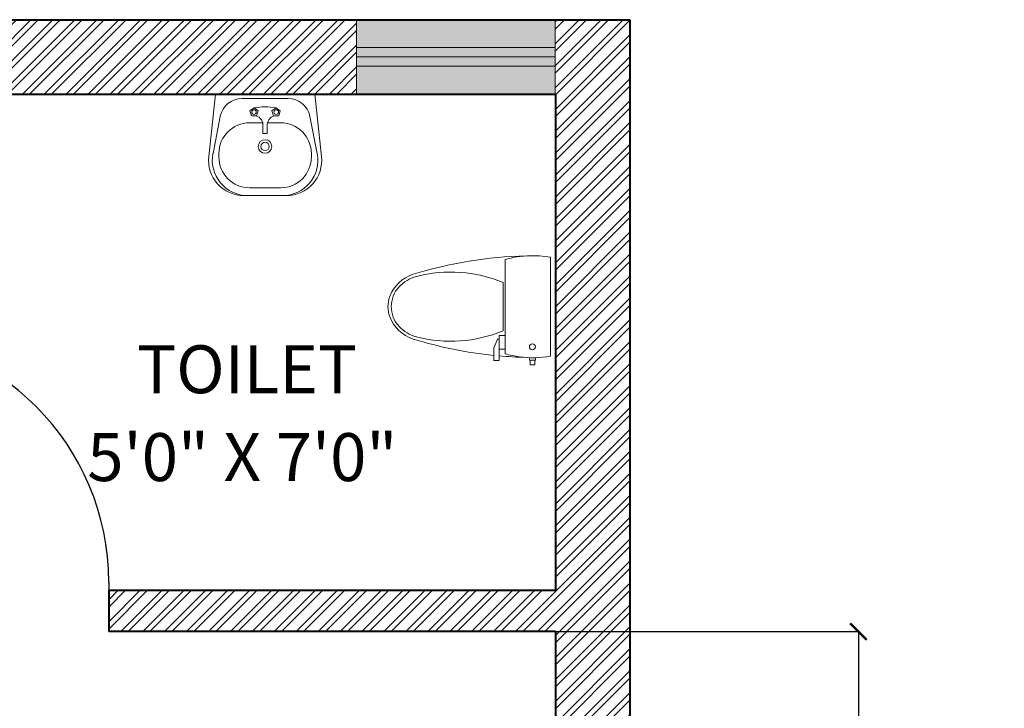
# Model space of a CAD drawing. Units: inches. Extents: x 528 to 2520, y -151 to 1354.
# Tile 41 of 41: x 2383 to 2502, y 815 to 898. Entities that reach past the tile are written whole.
import ezdxf

# ---------------------------------------------------------------- set-up
doc = ezdxf.new("R2010")
doc.units = ezdxf.units.IN
doc.header["$MEASUREMENT"] = 0
for name, color, linetype, lineweight in [('A-ANNO-DIMS', 2, 'Continuous', 18), ('A-AREA-IDEN', 7, 'Continuous', 18), ('A-Door', 150, 'Continuous', 25), ('A-ELEV-PROJ', 8, 'Continuous', 13), ('A-FLOR-FIXT', 9, 'Continuous', 18), ('A-WALL-PATT', 6, 'Continuous', 13), ('walls', 7, 'Continuous', 40), ('WINDOWS', 2, 'Continuous', 20)]:
    doc.layers.add(name, color=color, linetype=linetype, lineweight=lineweight)
doc.layers.add('A-GLAZ-PATT', color=152, linetype='Continuous', lineweight=13, true_color=0x2776bb)
doc.styles.get("Standard").update_dxf_attribs({"font": 'arial.ttf'})
doc.dimstyles.get("Standard").update_dxf_attribs({"dimtxt": 6, "dimasz": 2, "dimexe": 0.18, "dimexo": 0.0625, "dimgap": 0.09, "dimtad": 0, "dimtih": 1, "dimtoh": 1, "dimdec": 1, "dimzin": 0, "dimdsep": 46, "dimlunit": 3, "dimtxsty": 'Standard', "dimblk": 'ARCHTICK', "dimcen": 0.09, "dimadec": 0, "dimazin": 0, "dimtfac": 1, "dimtdec": 1, "dimtofl": 0, "dimtmove": 0, "dimatfit": 3, "dimfxl": 1, "dimtolj": 1, "dimtzin": 0, "dimarcsym": 0})

# ---------------------------------------------------------------- blocks, each defined once
blk = doc.blocks.new('toilet-7')
at = {"color": 0, "linetype": 'ByBlock'}
for p, q in [((0.2097, -0.02), (-0.2097, -0.02)), ((0.2151, -0.0677), (0.2097, -0.02)), ((0.2151, -0.1171), (0.2151, -0.0677)), ((-0.2457, -0.0874), (-0.2457, -0.1068)), ((-0.2457, -0.0874), (-0.2257, -0.0874)), ((-0.2457, -0.1068), (-0.2257, -0.1068)), ((-0.2257, -0.0846), (-0.2257, -0.1096)), ((-0.2257, -0.0846), (-0.2157, -0.0846)), ((-0.2257, -0.1096), (-0.2154, -0.1096)), ((0.2099, -0.164), (0.2151, -0.1171)), ((0.1991, -0.2124), (0.2099, -0.164)), ((-0.1213, -0.2374), (-0.2278, -0.2374)), ((-0.2278, -0.2374), (-0.2278, -0.2599)), ((0.1991, -0.2124), (-0.1991, -0.2124)), ((-0.1803, -0.2374), (-0.1803, -0.2124)), ((-0.1759, -0.2599), (-0.1379, -0.2451)), ((-0.1379, -0.2451), (-0.1379, -0.2374)), ((-0.1213, -0.2374), (-0.1213, -0.2124)), ((-0.1023, -0.2212), (0.1023, -0.2212)), ((-0.1759, -0.2599), (-0.2278, -0.2599))]:
    blk.add_line(p, q, dxfattribs=at)
blk.add_circle((-0.1696, -0.0971), 0.0125, dxfattribs=at)
for centre, radius, start, end in [((0.2244, -0.0924), 0.4402, 170.5377, 187.7399), ((1.517, -0.087), 1.7318, 181.2224, 184.9822), ((-1.517, -0.087), 1.7318, 342.7523, 358.7776), ((0.2244, -0.0924), 0.4402, 187.7399, 195.822), ((0.4258, -0.4413), 0.5721, 157.3737, 194.7786), ((-0.4258, -0.4413), 0.5721, 345.2214, 22.6263), ((1.517, -0.087), 1.7318, 185.7323, 197.2477), ((0.0116, -0.5544), 0.1554, 197.2477, 249.5476), ((0.0221, -0.5478), 0.1546, 194.7786, 226.8543), ((-0.0116, -0.5544), 0.1554, 290.4524, 342.7523), ((-0.0221, -0.5478), 0.1546, 313.1457, 345.2214), ((0, -0.5713), 0.1223, 226.8543, 313.1457), ((0, -0.5854), 0.1223, 249.5476, 290.4524)]:
    blk.add_arc(centre, radius, start, end, dxfattribs=at)
blk = doc.blocks.new('BASIN-WITH-TAP')
for p, q in [((0.84, 12.27), (0.02, 4.73)), ((12.84, 12.27), (0.84, 12.27)), ((12.84, 12.27), (13.66, 4.73)), ((9.64, 11.73), (4.05, 11.73)), ((1.43, 9.58), (0.55, 5.09)), ((5, 10.24), (5.51, 10.61)), ((5.2, 9.64), (5, 10.24)), ((5.24, 10.1), (5.2, 10.1)), ((5.24, 9.64), (5.51, 9.64)), ((5.51, 10.61), (6.02, 10.24)), ((6.02, 10.24), (5.82, 9.64)), ((8.18, 10.61), (7.67, 10.24)), ((7.67, 10.24), (7.86, 9.64)), ((8.68, 10.24), (8.18, 10.61)), ((8.49, 9.64), (8.18, 9.64)), ((8.44, 10.1), (8.49, 10.1)), ((8.49, 9.64), (8.68, 10.24)), ((12.26, 9.58), (13.14, 5.09)), ((4.98, 8.8), (6.58, 8.8)), ((6.58, 8.31), (6.58, 8.58)), ((8.71, 8.8), (7.11, 8.8)), ((7.11, 8.31), (7.11, 8.58)), ((6.58, 7.51), (6.58, 8.31)), ((6.58, 7.51), (7.11, 7.51)), ((7.11, 7.51), (7.11, 8.31)), ((1.24, 4.67), (1.24, 5.07)), ((12.44, 4.67), (12.44, 5.07)), ((4.73, 0), (8.96, 0)), ((6.84, 0.93), (4.98, 0.93)), ((6.84, 0.93), (8.71, 0.93))]:
    blk.add_line(p, q)
for centre, radius in [((5.5, 10.1), 0.277), ((8.19, 10.1), 0.277), ((6.84, 5.94), 0.821), ((6.84, 5.94), 0.507)]:
    blk.add_circle(centre, radius)
for centre, radius, start, end in [((4.05, 9.07), 2.67, 90, 168.8773), ((6.84, 4.01), 6.73, 78.5788, 101.4212), ((9.64, 9.07), 2.67, 11.1227, 90), ((5.51, 8.58), 1.07, 0, 90), ((8.18, 8.58), 1.07, 90, 180), ((4.98, 5.07), 3.73, 90, 180), ((8.71, 5.07), 3.73, 0, 90), ((4.73, 4.27), 4.27, 168.8773, 270), ((8.96, 4.27), 4.27, 270, 11.1227), ((4.27, 4.27), 4.27, 173.7966, 270), ((4.98, 4.67), 3.73, 180, 270), ((8.71, 4.67), 3.73, 270, 0), ((9.42, 4.27), 4.27, 270, 6.2034)]:
    blk.add_arc(centre, radius, start, end)
blk = doc.blocks.new('DOOR-SWING-30')
for p, q in [((0, 6), (0, 0)), ((30, 6), (30, 0))]:
    blk.add_line(p, q)
blk.add_lwpolyline([(0, 6), (0, 36), (1.75, 36), (1.75, 6)], close=True)
blk.add_arc((0, 6), 30, 0, 90)
blk = doc.blocks.new('WINDOW-24x9-PLAN')
for p, q in [((0, 5.63), (24, 5.63)), ((0, 4.5), (24, 4.5)), ((0, 3.37), (24, 3.37))]:
    blk.add_line(p, q)
blk.add_lwpolyline([(0, 9), (24, 9), (24, 0), (0, 0)], close=True)
blk = doc.blocks.new('_ArchTick')
at = {"color": 0, "linetype": 'ByBlock', "const_width": 0.15}
blk.add_lwpolyline([(-0.5, -0.5), (0.5, 0.5)], dxfattribs=at)
blk = doc.blocks.new('*D98')
at = {"layer": 'A-ANNO-DIMS', "color": 0, "lineweight": -2, "transparency": 16777216}
for p, q in [((2448.07, 823.94), (2484.84, 823.94)), ((2484.66, 823.94), (2484.66, 791.26)), ((2484.66, 752.2), (2484.66, 784.88)), ((2457.07, 752.2), (2484.84, 752.2))]:
    blk.add_line(p, q, dxfattribs=at)
at = {"layer": 'Defpoints', "color": 0, "transparency": 16777216}
for p in [(2448.01, 823.94), (2484.66, 823.94), (2457.01, 752.2)]:
    blk.add_point(p, dxfattribs=at)
at = {"layer": 'A-ANNO-DIMS', "color": 0, "lineweight": -2, "transparency": 16777216, "xscale": 2, "yscale": 2, "zscale": 2}
for p, rotation in [((2484.66, 823.94), 90), ((2484.66, 752.2), 270)]:
    blk.add_blockref('_ArchTick', p, dxfattribs=dict(at, rotation=rotation))
at = {"layer": 'A-ANNO-DIMS', "color": 0, "transparency": 16777216, "insert": (2484.66, 788.07), "char_height": 6, "attachment_point": 5}
blk.add_mtext('\\A1;5\'-11 1/2"', dxfattribs=at)

msp = doc.modelspace()

# ---------------------------------------------------------------- hatches: boundary and pattern name
at = {"layer": 'A-GLAZ-PATT'}
h = msp.add_hatch(color=256, dxfattribs=at)
h.dxf.hatch_style = 1
h.paths.add_polyline_path([(2447.97, 894.57), (2423.97, 894.57), (2423.97, 893.44), (2447.97, 893.44)])
h.paths.add_polyline_path([(2447.97, 893.44), (2423.97, 893.44), (2423.97, 892.31), (2447.97, 892.31)])
h.paths.add_polyline_path([(2447.97, 897.94), (2423.97, 897.94), (2423.97, 894.57), (2447.97, 894.57)])
h.paths.add_polyline_path([(2447.97, 892.31), (2423.97, 892.31), (2423.97, 888.94), (2447.97, 888.94)])
at = {"layer": 'A-WALL-PATT'}
h = msp.add_hatch(dxfattribs=at)
h.set_pattern_fill('ANSI32', color=256, scale=5)
h.set_pattern_definition([(45, (1571.3155, -419.1643), (-1.3258252, 1.3258252), []), (45, (1572.1993, -419.1643), (-1.3258252, 1.3258252), [])])
h.paths.add_polyline_path([(2167.01, 744.69), (2158.01, 744.69), (2158.01, 549.94), (2169.56, 549.94), (2174.56, 549.94), (2174.56, 554.94), (2167.01, 554.94), (2167.01, 662.94), (2263.01, 662.94), (2263.01, 667.94), (2263.01, 686.94), (2269.01, 686.94), (2269.01, 691.94), (2258.01, 691.94), (2258.01, 667.94), (2167.01, 667.94)])
h.paths.add_polyline_path([(2260.02, 554.94), (2222.56, 554.94), (2222.56, 549.94), (2260.02, 549.94)])
h.paths.add_polyline_path([(2457.01, 752.2), (2448.01, 752.2), (2448.01, 691.94), (2358.01, 691.94), (2358.01, 686.94), (2448.01, 686.94), (2448.01, 554.94), (2358.01, 554.94), (2358.01, 549.94), (2448.01, 549.94), (2448.01, 405.94), (2406.01, 405.94), (2406.01, 396.94), (2457.01, 396.94)])
h.paths.add_polyline_path([(2457.01, 897.94), (2447.97, 897.94), (2447.97, 888.94), (2448.01, 888.94), (2448.01, 828.94), (2394.01, 828.94), (2394.01, 823.94), (2448.01, 823.94), (2448.01, 800.2), (2457.01, 800.2)])
h.paths.add_polyline_path([(2423.97, 897.94), (2359.01, 897.94), (2359.01, 828.94), (2355.58, 828.94), (2355.58, 823.94), (2364.01, 823.94), (2364.01, 829.94), (2364.01, 888.94), (2423.97, 888.94)])
h.paths.add_polyline_path([(2256.01, 897.94), (2191.01, 897.94), (2191.01, 888.94), (2251.01, 888.94), (2251.01, 828.94), (2251.01, 823.94), (2256.01, 823.94), (2256.01, 829.08)])
h.paths.add_polyline_path([(2167.01, 888.94), (2167.01, 897.94), (2158.01, 897.94), (2158.01, 792.69), (2167.01, 792.69), (2167.01, 823.94), (2221.01, 823.94), (2221.01, 828.94), (2167.01, 828.94)])
h.paths.add_polyline_path([(2316.01, 549.94), (2316.01, 554.94), (2296.02, 554.94), (2296.02, 549.94), (2311.01, 549.94), (2311.01, 455.12), (2316.01, 455.12)])
h.paths.add_polyline_path([(2311.01, 549.94), (2299.01, 549.94), (2299.01, 545.95), (2302.05, 545.95), (2302.05, 542.51), (2305.75, 542.51), (2305.75, 538.08), (2311.01, 538.08)], flags=17)
h.paths.add_polyline_path([(2358.01, 405.94), (2316.01, 405.94), (2316.01, 413.12), (2311.01, 413.12), (2311.01, 396.94), (2358.01, 396.94)])

# ---------------------------------------------------------------- linework, layer by layer
at = {"layer": 'A-ELEV-PROJ'}
msp.add_line((2457.01, 360.94), (2457.01, 897.94), dxfattribs=at)
at = {"layer": 'walls'}
for p, q in [((2359.01, 897.94), (2457.01, 897.94)), ((2457.01, 897.94), (2457.01, 396.94)), ((2364.01, 888.94), (2448.01, 888.94)), ((2448.01, 888.94), (2448.01, 828.94)), ((2394.01, 828.94), (2448.01, 828.94)), ((2394.01, 828.94), (2394.01, 823.94)), ((2448.01, 823.94), (2394.01, 823.94)), ((2448.01, 823.94), (2448.01, 691.94))]:
    msp.add_line(p, q, dxfattribs=at)

# ---------------------------------------------------------------- block references
at = {"layer": 'A-Door'}
msp.add_blockref('DOOR-SWING-30', (2364.01, 823.94), dxfattribs=at)
at = {"layer": 'A-FLOR-FIXT'}
msp.add_blockref('BASIN-WITH-TAP', (2406.07, 876.67), dxfattribs=at)
at = {"layer": 'A-FLOR-FIXT', "xscale": -28.60654769571749, "yscale": 28.60654769571749, "zscale": 28.60654769571749, "rotation": 270}
msp.add_blockref('toilet-7', (2448.01, 863.24), dxfattribs=at)
at = {"layer": 'WINDOWS'}
msp.add_blockref('WINDOW-24x9-PLAN', (2423.97, 888.94), dxfattribs=at)

# ---------------------------------------------------------------- texts
at = {"layer": 'A-AREA-IDEN'}
for s, height, p in [('TOILET', 5.793, (2397.43, 852.77)), ('5\'0" X 7\'0"', 5.7926, (2391.41, 842.15))]:
    msp.add_text(s, height=height, dxfattribs=at).set_placement(p)

# ---------------------------------------------------------------- dimensions: what is measured, and where the dimension line sits
at = {"layer": 'A-ANNO-DIMS'}
dim = msp.add_linear_dim(base=(2484.66, 823.94), p1=(2457.01, 752.2), p2=(2448.01, 823.94), angle=90, dimstyle='Standard', override={"dimdec": 1, "dimlfac": 1, "dimrnd": 0, "dimzin": 1, "dimdsep": 46, "dimlunit": 4, "dimfrac": 2}, dxfattribs=at)
dim.commit()
dim.dimension.update_dxf_attribs({"geometry": '*D98', "text_midpoint": (2484.66, 788.07)})

doc.saveas('drawing.dxf')
